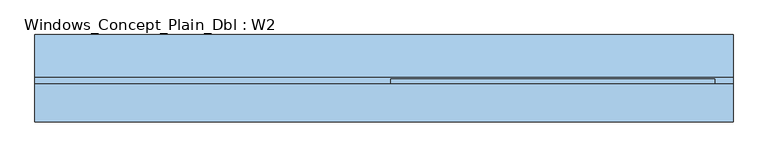
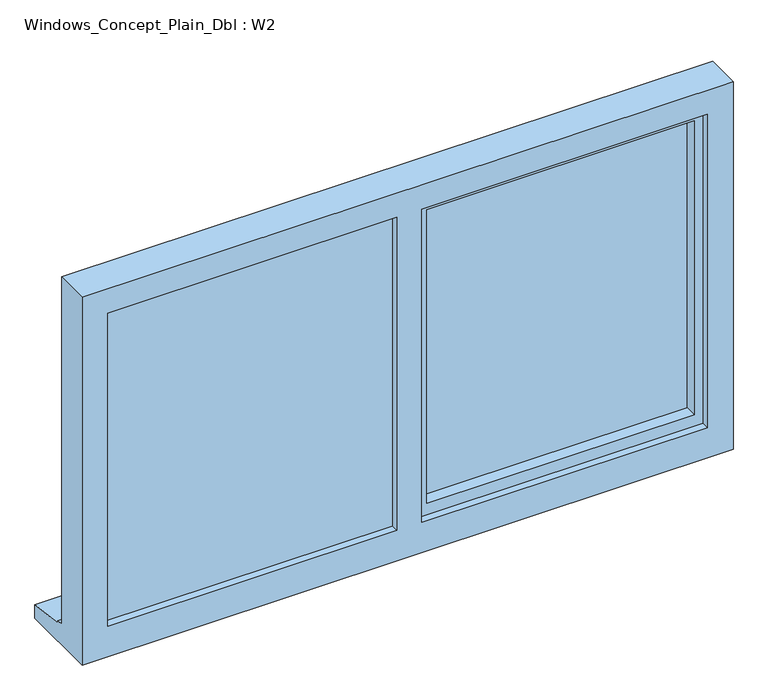
"""IFC4 building model written with IfcOpenShell, lengths in millimetres: window geometry, Windows_Concept_Plain_Dbl : W2."""

from ifc_helpers import new_model, si_unit, frame, origin, place, context, project, spatial, polyline, outline, extrude, faceted_brep, source, transform, mapped, element, save


def windows_concept_plain_dbl_w2_969b2eef(model_context):
    return source(origin(), model_context, "Body", "SolidModel", [
        faceted_brep([(-270.0, 22.9965678, 2070.0), (-270.0, 99.5435732, 2070.0), (-270.0, 99.5435732, 1263.0), (-270.0, 22.9965678, 1263.0), (-230.0, 51.9965678, 2030.0), (-230.0, 22.9965678, 2030.0), (-230.0, 22.9965678, 1303.0), (-230.0, 51.9965678, 1303.0), (-240.0, 75.9965678, 2040.0), (-240.0, 51.9965678, 2040.0), (-240.0, 51.9965678, 1293.0), (-240.0, 75.9965678, 1293.0), (-230.0, 99.5435732, 2030.0), (-230.0, 75.9965678, 2030.0), (-230.0, 75.9965678, 1303.0), (-230.0, 99.5435732, 1303.0), (437.0, 99.5435732, 1263.0), (437.0, 22.9965678, 1263.0), (397.0, 22.9965678, 1303.0), (397.0, 51.9965678, 1303.0), (407.0, 51.9965678, 1293.0), (407.0, 75.9965678, 1293.0), (397.0, 75.9965678, 1303.0), (397.0, 99.5435732, 1303.0), (437.0, 99.5435732, 2070.0), (437.0, 22.9965678, 2070.0), (397.0, 22.9965678, 2030.0), (397.0, 51.9965678, 2030.0), (407.0, 51.9965678, 2040.0), (407.0, 75.9965678, 2040.0), (397.0, 75.9965678, 2030.0), (397.0, 99.5435732, 2030.0)], [[[0, 1, 2, 3]], [[4, 5, 6, 7]], [[8, 9, 10, 11]], [[12, 13, 14, 15]], [[3, 2, 16, 17]], [[7, 6, 18, 19]], [[11, 10, 20, 21]], [[15, 14, 22, 23]], [[17, 16, 24, 25]], [[19, 18, 26, 27]], [[21, 20, 28, 29]], [[23, 22, 30, 31]], [[1, 24, 16, 2], [15, 23, 31, 12]], [[25, 24, 1, 0]], [[3, 17, 25, 0], [5, 26, 18, 6]], [[27, 26, 5, 4]], [[9, 28, 20, 10], [7, 19, 27, 4]], [[29, 28, 9, 8]], [[11, 21, 29, 8], [13, 30, 22, 14]], [[31, 30, 13, 12]]]),
        extrude(outline(polyline([(2050.0, -310.0), (2070.0, -310.0), (2070.0, -1007.0), (1263.0, -1007.0), (1263.0, -310.0), (1283.0, -310.0), (1283.0, -987.0), (2050.0, -987.0), (2050.0, -310.0)])), frame((0.0, 46.9965678, 0.0), z_axis=(0.0, 1.0, 0.0), x_axis=(0.0, 0.0, 1.0)), (0.0, 0.0, 1.0), 41.0),
        faceted_brep([(477.0, 4.9965678, 2110.0), (-1047.0, 4.9965678, 2110.0), (-1047.0, 4.9965678, 1200.0), (477.0, 4.9965678, 1200.0), (417.0, 4.9965678, 2050.0), (417.0, 4.9965678, 1275.0), (-252.0, 4.9965678, 1275.0), (-252.0, 4.9965678, 2050.0), (-310.0, 4.9965678, 2050.0), (-310.0, 4.9965678, 1275.0), (-987.0, 4.9965678, 1275.0), (-987.0, 4.9965678, 2050.0), (-1047.0, 87.9965678, 2110.0), (-1047.0, 87.9965678, 1251.0), (-1047.0, 102.9965678, 1249.68767), (-1047.0, 102.9965678, 1244.7449676), (-1047.0, 195.9565678, 1233.8088847), (-1047.0, 195.9565678, 1200.0), (477.0, 87.9965678, 2110.0), (477.0, 87.9965678, 1251.0), (-1007.0, 87.9965678, 2070.0), (-1007.0, 87.9965678, 1263.0), (-310.0, 87.9965678, 1263.0), (-310.0, 87.9965678, 2070.0), (-270.0, 87.9965678, 2070.0), (-270.0, 87.9965678, 1263.0), (437.0, 87.9965678, 1263.0), (437.0, 87.9965678, 2070.0), (-1007.0, 22.9965678, 2070.0), (-1007.0, 22.9965678, 1263.0), (-300.0, 22.9965678, 2070.0), (-300.0, 22.9965678, 1263.0), (-310.0, 22.9965678, 2050.0), (-987.0, 22.9965678, 2050.0), (-987.0, 22.9965678, 1275.0), (-310.0, 22.9965678, 1275.0), (-270.0, 22.9965678, 2070.0), (437.0, 22.9965678, 2070.0), (437.0, 22.9965678, 1263.0), (-270.0, 22.9965678, 1263.0), (417.0, 22.9965678, 2050.0), (-252.0, 22.9965678, 2050.0), (-252.0, 22.9965678, 1275.0), (417.0, 22.9965678, 1275.0), (-310.0, 46.9965678, 2070.0), (-300.0, 46.9965678, 2070.0), (477.0, 195.9565678, 1200.0), (477.0, 195.9565678, 1233.8088847), (477.0, 102.9965678, 1244.7449676), (477.0, 102.9965678, 1249.68767), (-300.0, 46.9965678, 1263.0), (-310.0, 46.9965678, 1263.0)], [[[0, 1, 2, 3], [4, 5, 6, 7], [8, 9, 10, 11]], [[2, 1, 12, 13, 14, 15, 16, 17]], [[13, 12, 18, 19], [20, 21, 22, 23], [24, 25, 26, 27]], [[21, 20, 28, 29]], [[28, 30, 31, 29], [32, 33, 34, 35]], [[36, 37, 38, 39], [40, 41, 42, 43]], [[33, 11, 10, 34]], [[1, 0, 18, 12]], [[28, 20, 23, 44, 45, 30]], [[27, 37, 36, 24]], [[11, 33, 32, 8]], [[40, 4, 7, 41]], [[19, 18, 0, 3, 46, 47, 48, 49]], [[27, 26, 38, 37]], [[4, 40, 43, 5]], [[45, 50, 31, 30]], [[50, 45, 44, 51]], [[51, 44, 23, 22]], [[25, 24, 36, 39]], [[41, 7, 6, 42]], [[8, 32, 35, 9]], [[46, 3, 2, 17]], [[47, 46, 17, 16]], [[48, 47, 16, 15]], [[49, 48, 15, 14]], [[19, 49, 14, 13]], [[22, 21, 29, 31, 50, 51]], [[26, 25, 39, 38]], [[6, 5, 43, 42]], [[35, 34, 10, 9]]]),
        extrude(outline(polyline([(-1007.0, 46.9965678), (-300.0, 46.9965678), (-300.0, 22.9965678), (-1007.0, 22.9965678), (-1007.0, 46.9965678)])), frame((0.0, 0.0, 1263.0), z_axis=(0.0, 0.0, 1.0), x_axis=(1.0, 0.0, 0.0)), (0.0, 0.0, 1.0), 807.0),
        extrude(outline(polyline([(407.0, 51.9965678), (-240.0, 51.9965678), (-240.0, 75.9965678), (407.0, 75.9965678), (407.0, 51.9965678)])), frame((0.0, 0.0, 1293.0), z_axis=(0.0, 0.0, 1.0), x_axis=(1.0, 0.0, 0.0)), (0.0, 0.0, 1.0), 747.0),
    ])


if __name__ == "__main__":
    model = new_model("IFC4")
    model_context = context("Model", 3, world=origin())
    ifc_project = project(units=[si_unit("LENGTHUNIT", "METRE", prefix="MILLI")], contexts=[model_context])
    site = spatial("IfcSite", under=ifc_project)
    building = spatial("IfcBuilding", under=site)
    placement = place(None, origin())
    windows_concept_plain_dbl_w2_shape = windows_concept_plain_dbl_w2_969b2eef(model_context)
    element("IfcWindow", 1, ObjectType="Windows_Concept_Plain_Dbl : W2", at=placement, inside=building, context=model_context, shape_type="MappedRepresentation", body=[
        mapped(windows_concept_plain_dbl_w2_shape, transform((0.0, 0.0, 0.0), x_axis=(1.0, 0.0, 0.0), y_axis=(0.0, 1.0, 0.0), z_axis=(0.0, 0.0, 1.0))),
    ])
    save(model, "model.ifc")

# Revit data of these elements
# Type "Windows_Concept_Plain_Dbl : W2"
#   Type Mark = "57"
#   Operation = "DoublePanelVertical"
#   Construction Type Id = "GSP4R"
#   Manufacturer = "Revit"
#   Keynote = "L10"
#   Analytic Construction = "1/8 in Pilkington single glazing"
#   Visual Light Transmittance = 0.9
#   Solar Heat Gain Coefficient = 0.78
#   Rough Width = 1524 mm
#   Rough Height = 910 mm
#   Height = 910 mm
#   Width = 1524 mm
#   Heat Transfer Coefficient (U) = 3.6886 W/(m²·K)
#   FrameOffset - External = 50 mm
#   Default Head Height = 2110 mm
#   Vis - Cavity Closers = yes
#   Define Thermal Properties by = 1
#   Material Trim = Window Frame
#   Material Glass = Glass
#   Material Frame = Window Frame
#   Wall Closure = (empty or 0)
# Element 1 (IfcWindow, "Windows_Concept_Plain_Dbl : W2")
#   Materials on its faces: "Window Frame", "Glass"
# Materials
#   "Window Frame": colour RGB 249 249 249, transparency 0, Keynote = "L10", Cost = 0
#   "Glass": class "Glass", colour RGB 0 128 192, transparency 0.9, Description = "Soda Lime Glass", Cost = 0
